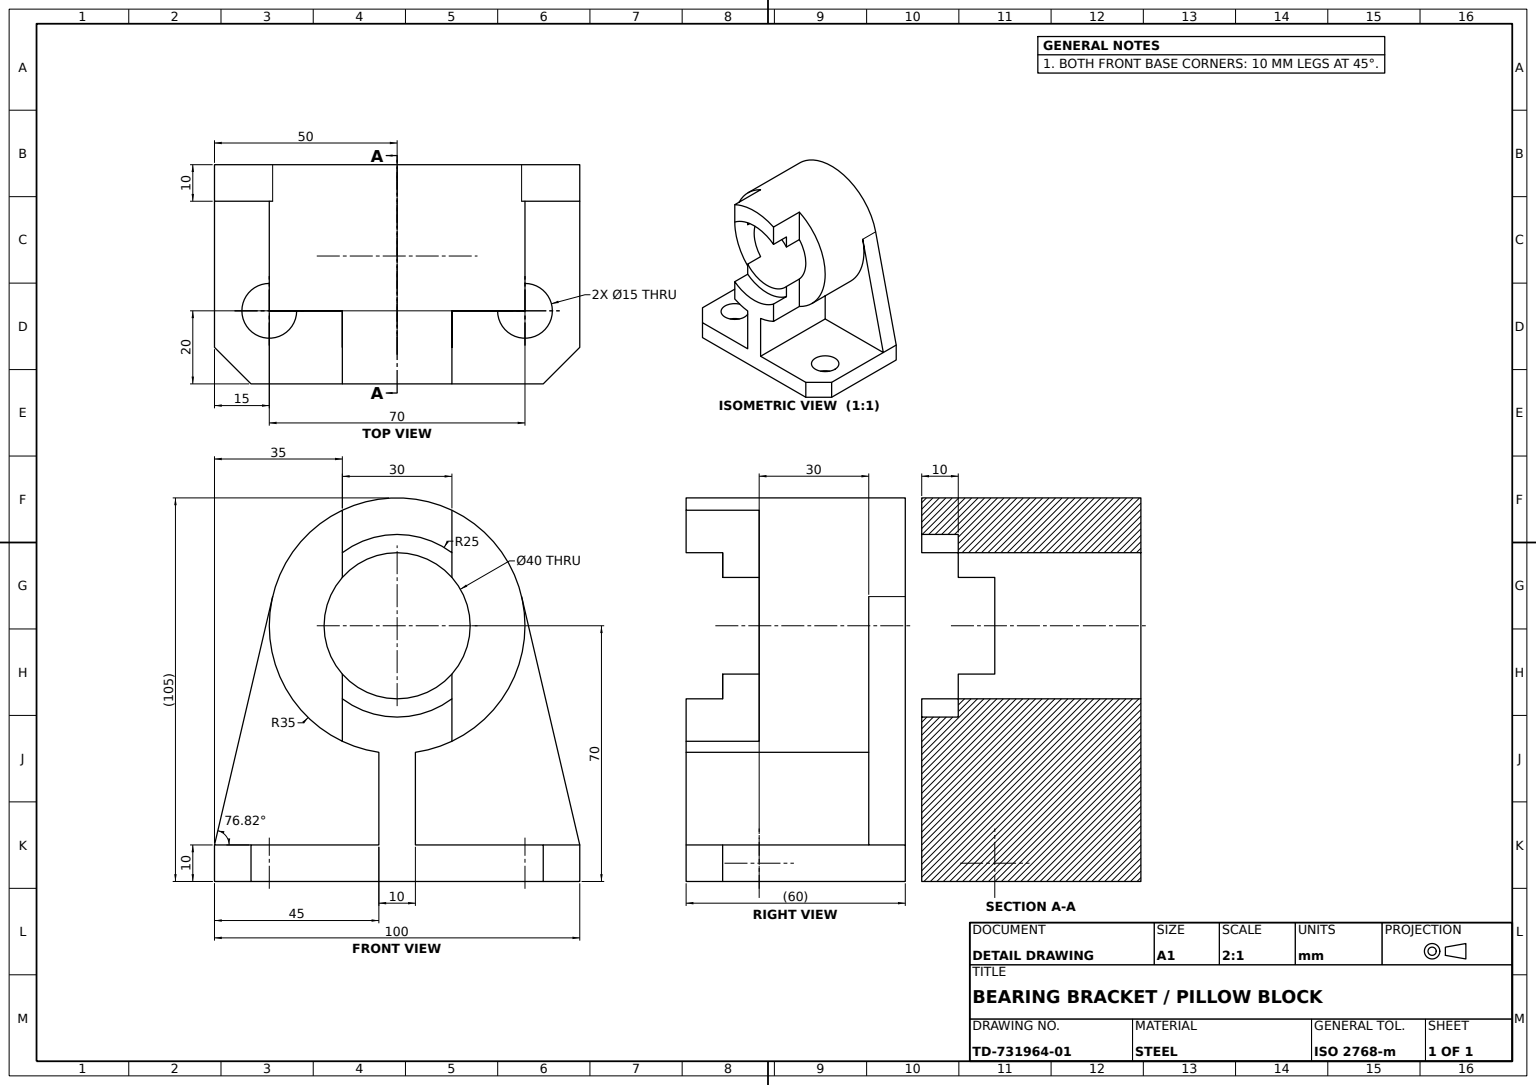
from build123d import *

# Parameters (mm, degrees)
BACK_PLATE_DEPTH        = 10
BASE_PLATE_DEPTH        = 10
HOUSING_BOSS_DEPTH      = 50
MOUNTING_HOLES_REACH    = 124.984
MOUNTING_HOLES_SKETCH_R = 7.5
HOUSING_SLOT_PROFILE_W  = 28.353660078
HOUSING_SLOT_PROFILE_H  = 63.245553204
HOUSING_SLOT_CUT_DEPTH  = 20


with BuildPart() as part:
    # Back Plate Profile → Back Plate (new body)
    with BuildSketch(Plane(origin=(0, 0, 0), x_dir=(0, 0, -1), z_dir=(1, 0, 0))):
        with BuildLine():
            Line((-50, -70), (50, -70))
            Line((50, -70), (50, -60))
            Line((50, -60), (34.077790239, 7.981491866))
            ThreePointArc((34.077790239, 7.981491866), (0, 35), (-34.077790239, 7.981491866))
            Line((-34.077790239, 7.981491866), (-50, -60))
            Line((-50, -60), (-50, -70))
        make_face()
    extrude(amount=BACK_PLATE_DEPTH)

    # Base Plate Profile → Base Plate (add)
    with BuildSketch(Plane.XZ.offset(70)):
        Polygon((10, 50), (50, 50), (60, 40), (60, -40), (50, -50), (10, -50), align=None)
    extrude(amount=-BASE_PLATE_DEPTH)

    # Housing Boss Profile → Housing Boss (add)
    with BuildSketch(Plane(origin=(10, 0, 0), x_dir=(0, 0, -1), z_dir=(1, 0, 0))):
        with BuildLine():
            Line((-5, -34.641016151), (-5, -60))
            Line((-5, -60), (5, -60))
            Line((5, -60), (5, -34.641016151))
            ThreePointArc((5, -34.641016151), (0, 35), (-5, -34.641016151))
        make_face()
    extrude(amount=HOUSING_BOSS_DEPTH)

    # Mounting Holes Sketch → Mounting Holes (cut, up to next)
    with BuildSketch(Plane(origin=(0, -60, 0), x_dir=(1, 0, 0), z_dir=(0, 1, 0)), mode=Mode.PRIVATE) as mounting_holes_sk1:
        with Locations(Location((40, 35, 0), (0, 0, 270))):
            Circle(MOUNTING_HOLES_SKETCH_R)
    mounting_holes_tool1 = extrude(mounting_holes_sk1.sketch, amount=-MOUNTING_HOLES_REACH, mode=Mode.PRIVATE) & part.part
    # Mounting Holes Sketch → Mounting Holes (cut, up to next)
    with BuildSketch(Plane(origin=(0, -60, 0), x_dir=(1, 0, 0), z_dir=(0, 1, 0)), mode=Mode.PRIVATE) as mounting_holes_sk2:
        with Locations(Location((40, -35, 0), (0, 0, 270))):
            Circle(MOUNTING_HOLES_SKETCH_R)
    mounting_holes_tool2 = extrude(mounting_holes_sk2.sketch, amount=-MOUNTING_HOLES_REACH, mode=Mode.PRIVATE) & part.part
    add(mounting_holes_tool1.solids().sort_by_distance((40, -60, -35))[0], mode=Mode.SUBTRACT)
    add(mounting_holes_tool2.solids().sort_by_distance((40, -60, 35))[0], mode=Mode.SUBTRACT)

    # Gland Bore Profile → Gland Bore (revolve, cut)
    with BuildSketch(Plane.XY, mode=Mode.PRIVATE) as gland_bore_sk:
        Polygon((0, 0), (60, 0), (60, 25), (50, 25), (50, 20), (40, 20), (0, 20), align=None)
    revolve(gland_bore_sk.sketch.rotate(Axis((0, 0, 0), (1, 0, 0)), 90), axis=Axis((0, 0, 0), (1, 0, 0)), mode=Mode.SUBTRACT)

    # Housing Slot Profile → Housing Slot Cut (cut)
    with BuildSketch(Plane(origin=(60, 0, 0), x_dir=(0, 0, -1), z_dir=(1, 0, 0))):
        with Locations((-29.176830039, 0)):
            Rectangle(HOUSING_SLOT_PROFILE_W, HOUSING_SLOT_PROFILE_H)
        with Locations((29.176830039, 0)):
            Rectangle(HOUSING_SLOT_PROFILE_W, HOUSING_SLOT_PROFILE_H)
    extrude(amount=-HOUSING_SLOT_CUT_DEPTH, mode=Mode.SUBTRACT)


solid = part.part
